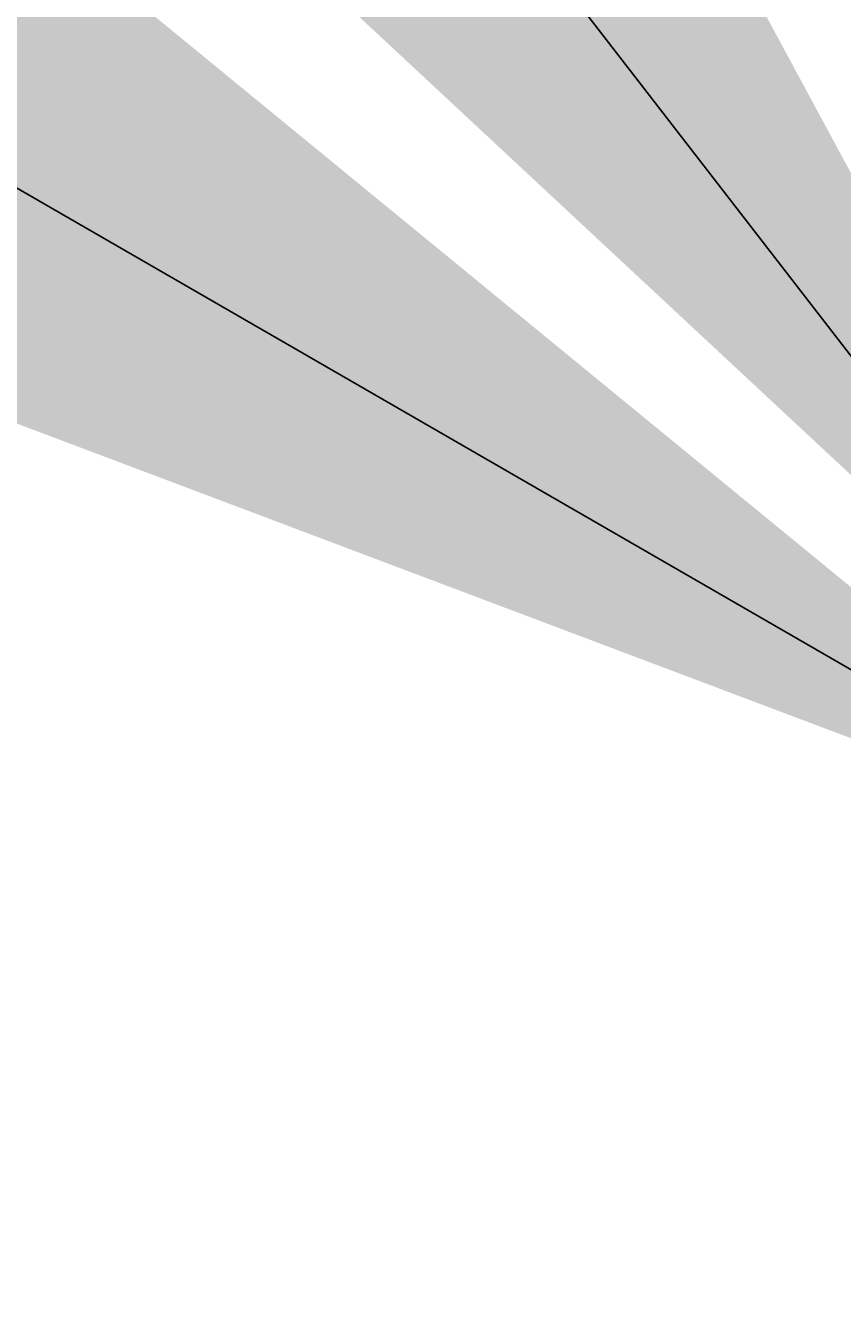
# Model space of a CAD drawing. Units: inches. Extents: x -9413 to 9703, y -9719 to 9096.
# Tile 1 of 1: x -993 to -250, y -311 to 865. Entities that reach past the tile are written whole.
import ezdxf
from ezdxf import colors
from ezdxf.entities.mleader import LeaderData, LeaderLine
from ezdxf.math import Vec2, Vec3

# ---------------------------------------------------------------- set-up
doc = ezdxf.new("R2010")
doc.units = ezdxf.units.IN
doc.header["$MEASUREMENT"] = 0
doc.layers.add('M-ANNO-TEXT', color=7, linetype='Continuous', lineweight=18)
doc.styles.get("Standard").update_dxf_attribs({"font": 'arial.ttf'})

msp = doc.modelspace()

# ---------------------------------------------------------------- leaders
at = {"layer": 'M-ANNO-TEXT'}
ml = msp.add_multileader_mtext('Standard', dxfattribs=at)
ml.set_content('steam drum', color=256)
ml.set_leader_properties()
ml.build(insert=Vec2(0, 0))
ml.multileader.update_dxf_attribs({"dogleg_length": 0.36, "arrow_head_size": 10000, "scale": 10})
ctx = ml.context
ctx.base_point, ctx.scale, ctx.char_height, ctx.arrow_head_size, ctx.landing_gap_size, ctx.plane_origin = Vec3(1.078100315116472, 187.1657656808087), 10, 5.4, 10000, 0.9, Vec3(56.53630785249729, 178.1917761520126)
ctx.text_align_type = 2
notes = []
notes.append((ctx, [(0, (1, 1, 0), (49.60206616053652, 187.1657656808087), (-1, 0), 7.616326009130828, [(0, [(56.5363078524973, 178.1917761520126)], 0, [])])]))
ctx.mtext.insert, ctx.mtext.alignment, ctx.mtext.flow_direction = Vec3(41.08574015140569, 189.9099675907678), 3, 5
ml = msp.add_multileader_mtext('Standard', dxfattribs=at)
ml.set_content('Boiler', color=256)
ml.set_leader_properties()
ml.build(insert=Vec2(0, 0))
ml.multileader.update_dxf_attribs({"dogleg_length": 0.36, "arrow_head_size": 10000, "scale": 10})
ctx = ml.context
ctx.base_point, ctx.scale, ctx.char_height, ctx.arrow_head_size, ctx.landing_gap_size, ctx.plane_origin = Vec3(31.04430257849453, 103.0991380116177), 10, 5.4, 10000, 0.9, Vec3(69.11352005531556, 99.3051261342938)
ctx.text_align_type = 2
notes.append((ctx, [(0, (1, 1, 0), (62.54209871927075, 103.0991380116177), (-1, 0), 10.86041551321825, [(0, [(69.11352005531556, 99.3051261342938)], 0, [])])]))
ctx.mtext.insert, ctx.mtext.alignment, ctx.mtext.flow_direction = Vec3(50.7816832060525, 105.8433399215768), 3, 5
ml = msp.add_multileader_mtext('Standard', dxfattribs=at)
ml.set_content('Air preheater', color=256)
ml.set_leader_properties()
ml.build(insert=Vec2(0, 0))
ml.multileader.update_dxf_attribs({"dogleg_length": 0.36, "arrow_head_size": 10000, "scale": 10})
ctx = ml.context
ctx.base_point, ctx.scale, ctx.char_height, ctx.arrow_head_size, ctx.landing_gap_size, ctx.plane_origin = Vec3(229.7079293124727, 37.30650895205824), 10, 5.4, 10000, 0.9, Vec3(241.9833706008503, 78.04556948044049)
notes.append((ctx, [(1, (1, 1, 0), (223.7048975654645, 37.30650895205824), (1, 0), 6.003031747008185, [(0, [(241.9833706008503, 78.04556948044049)], 0, [])])]))
ctx.mtext.insert, ctx.mtext.flow_direction = Vec3(230.6079293124727, 40.75609967511417), 5
for ctx, leaders in notes:
    for number, flags, end, landing, length, lines in leaders:
        leader = LeaderData()
        leader.index, (leader.has_last_leader_line, leader.has_dogleg_vector, leader.attachment_direction) = number, flags
        leader.last_leader_point, leader.dogleg_vector, leader.dogleg_length = Vec3(end), Vec3(landing), length
        for number, points, colour, breaks in lines:
            line = LeaderLine()
            line.index, line.vertices, line.color, line.breaks = number, Vec3.list(points), colors.encode_raw_color(colour), breaks
            leader.lines.append(line)
        ctx.leaders.append(leader)

doc.saveas('drawing.dxf')
